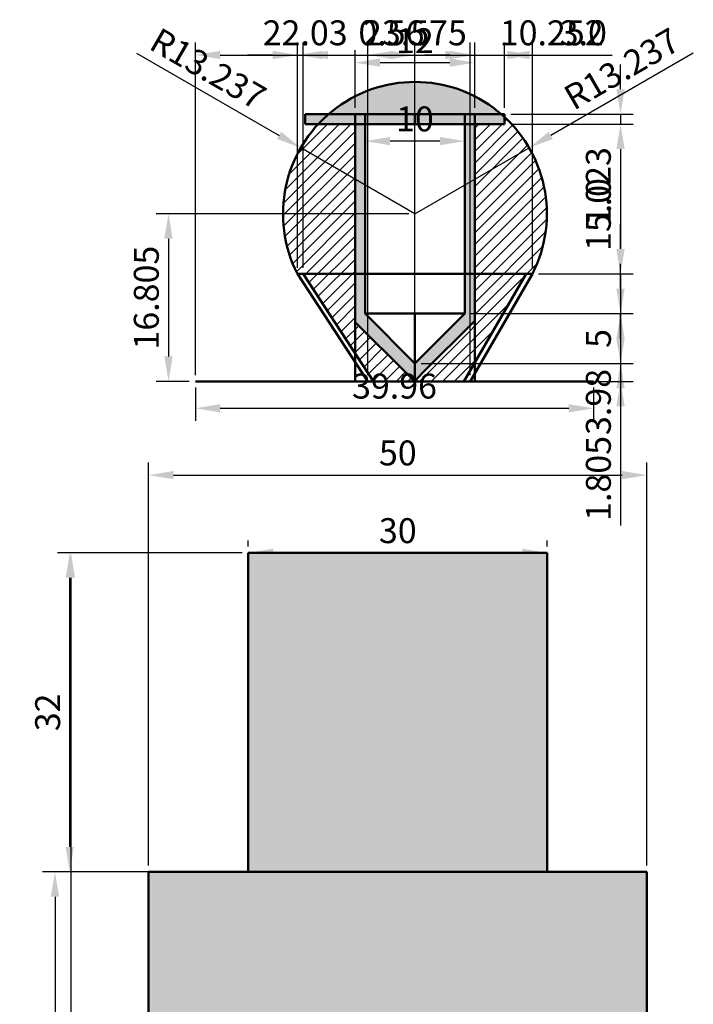
# Model space of a CAD drawing. Units: millimetres. Extents: x 1159 to 1466, y 1237 to 1440.
# Tile 2 of 6: x 1163 to 1230, y 1341 to 1440. Entities that reach past the tile are written whole.
import ezdxf

# ---------------------------------------------------------------- set-up
doc = ezdxf.new("R2010")
doc.units = ezdxf.units.MM
for name, color, linetype, lineweight in [('M-DIMS', 2, 'Continuous', 25), ('M-HATC', 8, 'Continuous', 18), ('M-OUTL', 7, 'Continuous', 50)]:
    doc.layers.add(name, color=color, linetype=linetype, lineweight=lineweight)
doc.styles.get("Standard").update_dxf_attribs({"font": 'arial.ttf'})
doc.dimstyles.new('ISO-25', dxfattribs={"dimtxt": 2.5, "dimasz": 2.5, "dimexe": 1.25, "dimexo": 0.625, "dimtad": 1, "dimtxsty": 'Standard', "dimcen": 2.5, "dimadec": 0, "dimazin": 0, "dimtfac": 1, "dimtmove": 0, "dimatfit": 3, "dimfxl": 1, "dimarcsym": 0})

# ---------------------------------------------------------------- blocks, each defined once
blk = doc.blocks.new('*D2')
at = {"layer": 'Defpoints', "color": 0, "transparency": 16777216}
for p in [(1208.23, 1435.45), (1196.23, 1430.28), (1208.23, 1430.28)]:
    blk.add_point(p, dxfattribs=at)
at = {"layer": 'M-DIMS', "color": 0, "lineweight": -2, "transparency": 16777216}
for p, q in [((1196.23, 1430.905), (1196.23, 1436.7)), ((1208.23, 1430.905), (1208.23, 1436.7)), ((1198.73, 1435.45), (1205.73, 1435.45))]:
    blk.add_line(p, q, dxfattribs=at)
at = {"layer": 'M-DIMS', "color": 0, "transparency": 16777216}
for points in [[(1198.73, 1435.867), (1198.73, 1435.034), (1196.23, 1435.45)], [(1205.73, 1435.867), (1205.73, 1435.034), (1208.23, 1435.45)]]:
    blk.add_solid(points, dxfattribs=at)
at = {"layer": 'M-DIMS', "color": 0, "transparency": 16777216, "insert": (1202.23, 1437.33), "char_height": 2.5, "attachment_point": 5}
blk.add_mtext('12', dxfattribs=at)
blk = doc.blocks.new('*D9')
at = {"layer": 'Defpoints', "color": 0, "transparency": 16777216}
for p in [(1185.51, 1386.27), (1215.51, 1386.27), (1215.51, 1386.27)]:
    blk.add_point(p, dxfattribs=at)
at = {"layer": 'M-DIMS', "color": 0, "lineweight": -2, "transparency": 16777216}
for p, q in [((1185.51, 1386.895), (1185.51, 1387.52)), ((1215.51, 1386.895), (1215.51, 1387.52)), ((1188.01, 1386.27), (1213.01, 1386.27))]:
    blk.add_line(p, q, dxfattribs=at)
at = {"layer": 'M-DIMS', "color": 0, "transparency": 16777216}
for points in [[(1188.01, 1386.687), (1188.01, 1385.854), (1185.51, 1386.27)], [(1213.01, 1386.687), (1213.01, 1385.854), (1215.51, 1386.27)]]:
    blk.add_solid(points, dxfattribs=at)
at = {"layer": 'M-DIMS', "color": 0, "transparency": 16777216, "insert": (1200.51, 1388.173), "char_height": 2.5, "attachment_point": 5}
blk.add_mtext('30', dxfattribs=at)
blk = doc.blocks.new('*D11')
at = {"layer": 'Defpoints', "color": 0, "transparency": 16777216}
for p in [(1167.601, 1386.27), (1185.51, 1386.27), (1185.51, 1354.27)]:
    blk.add_point(p, dxfattribs=at)
at = {"layer": 'M-DIMS', "color": 0, "lineweight": -2, "transparency": 16777216}
for p, q in [((1184.885, 1386.27), (1166.351, 1386.27)), ((1167.601, 1356.77), (1167.601, 1383.77)), ((1184.885, 1354.27), (1166.351, 1354.27))]:
    blk.add_line(p, q, dxfattribs=at)
at = {"layer": 'M-DIMS', "color": 0, "transparency": 16777216}
for points in [[(1167.185, 1383.77), (1168.018, 1383.77), (1167.601, 1386.27)], [(1167.185, 1356.77), (1168.018, 1356.77), (1167.601, 1354.27)]]:
    blk.add_solid(points, dxfattribs=at)
at = {"layer": 'M-DIMS', "color": 0, "transparency": 16777216, "insert": (1165.699, 1370.27), "char_height": 2.5, "attachment_point": 5, "rotation": 90}
blk.add_mtext('32', dxfattribs=at)
blk = doc.blocks.new('*D12')
at = {"layer": 'Defpoints', "color": 0, "transparency": 16777216}
for p in [(1175.51, 1354.27), (1166.114, 1320.27), (1175.51, 1320.27)]:
    blk.add_point(p, dxfattribs=at)
at = {"layer": 'M-DIMS', "color": 0, "lineweight": -2, "transparency": 16777216}
for p, q in [((1174.885, 1354.27), (1164.864, 1354.27)), ((1166.114, 1351.77), (1166.114, 1322.77)), ((1174.885, 1320.27), (1164.864, 1320.27))]:
    blk.add_line(p, q, dxfattribs=at)
at = {"layer": 'M-DIMS', "color": 0, "transparency": 16777216}
for points in [[(1165.697, 1351.77), (1166.53, 1351.77), (1166.114, 1354.27)], [(1165.697, 1322.77), (1166.53, 1322.77), (1166.114, 1320.27)]]:
    blk.add_solid(points, dxfattribs=at)
at = {"layer": 'M-DIMS', "color": 0, "transparency": 16777216, "insert": (1164.211, 1337.27), "char_height": 2.5, "attachment_point": 5, "rotation": 90}
blk.add_mtext('34', dxfattribs=at)
blk = doc.blocks.new('*D23')
at = {"layer": 'Defpoints', "color": 0, "transparency": 16777216}
for p in [(1185.51, 1386.27), (1167.71, 1260.27), (1190.51, 1260.27)]:
    blk.add_point(p, dxfattribs=at)
at = {"layer": 'M-DIMS', "color": 0, "lineweight": -2, "transparency": 16777216}
for p, q in [((1184.885, 1386.27), (1166.46, 1386.27)), ((1167.71, 1383.77), (1167.71, 1262.77)), ((1189.885, 1260.27), (1166.46, 1260.27))]:
    blk.add_line(p, q, dxfattribs=at)
at = {"layer": 'M-DIMS', "color": 0, "transparency": 16777216}
for points in [[(1167.293, 1383.77), (1168.127, 1383.77), (1167.71, 1386.27)], [(1167.293, 1262.77), (1168.127, 1262.77), (1167.71, 1260.27)]]:
    blk.add_solid(points, dxfattribs=at)
at = {"layer": 'M-DIMS', "color": 0, "transparency": 16777216, "insert": (1165.809, 1323.27), "char_height": 2.5, "attachment_point": 5, "rotation": 90}
blk.add_mtext('126', dxfattribs=at)
blk = doc.blocks.new('*D24')
at = {"layer": 'Defpoints', "color": 0, "transparency": 16777216}
for p in [(1225.51, 1394.07), (1175.51, 1354.27), (1225.51, 1354.27)]:
    blk.add_point(p, dxfattribs=at)
at = {"layer": 'M-DIMS', "color": 0, "lineweight": -2, "transparency": 16777216}
for p, q in [((1175.51, 1354.895), (1175.51, 1395.32)), ((1225.51, 1354.895), (1225.51, 1395.32)), ((1178.01, 1394.07), (1223.01, 1394.07))]:
    blk.add_line(p, q, dxfattribs=at)
at = {"layer": 'M-DIMS', "color": 0, "transparency": 16777216}
for points in [[(1178.01, 1394.487), (1178.01, 1393.654), (1175.51, 1394.07)], [(1223.01, 1394.487), (1223.01, 1393.654), (1225.51, 1394.07)]]:
    blk.add_solid(points, dxfattribs=at)
at = {"layer": 'M-DIMS', "color": 0, "transparency": 16777216, "insert": (1200.51, 1395.972), "char_height": 2.5, "attachment_point": 5}
blk.add_mtext('50', dxfattribs=at)
blk = doc.blocks.new('*D37')
at = {"layer": 'Defpoints', "color": 0, "transparency": 16777216}
for p in [(1202.23, 1420.28), (1177.501, 1403.475), (1180.201, 1403.475)]:
    blk.add_point(p, dxfattribs=at)
at = {"layer": 'M-DIMS', "color": 0, "lineweight": -2, "transparency": 16777216}
for p, q in [((1201.605, 1420.28), (1176.251, 1420.28)), ((1177.501, 1417.78), (1177.501, 1405.975)), ((1179.576, 1403.475), (1176.251, 1403.475))]:
    blk.add_line(p, q, dxfattribs=at)
at = {"layer": 'M-DIMS', "color": 0, "transparency": 16777216}
for points in [[(1177.085, 1417.78), (1177.918, 1417.78), (1177.501, 1420.28)], [(1177.085, 1405.975), (1177.918, 1405.975), (1177.501, 1403.475)]]:
    blk.add_solid(points, dxfattribs=at)
at = {"layer": 'M-DIMS', "color": 0, "transparency": 16777216, "insert": (1175.6, 1411.877), "char_height": 2.5, "attachment_point": 5, "rotation": 90}
blk.add_mtext('16.805', dxfattribs=at)
blk = doc.blocks.new('*D38')
at = {"layer": 'Defpoints', "color": 0, "transparency": 16777216}
for p in [(1180.201, 1403.475), (1220.161, 1403.475), (1220.161, 1400.775)]:
    blk.add_point(p, dxfattribs=at)
at = {"layer": 'M-DIMS', "color": 0, "lineweight": -2, "transparency": 16777216}
for p, q in [((1180.201, 1402.85), (1180.201, 1399.525)), ((1220.161, 1402.85), (1220.161, 1399.525)), ((1182.701, 1400.775), (1217.661, 1400.775))]:
    blk.add_line(p, q, dxfattribs=at)
at = {"layer": 'M-DIMS', "color": 0, "transparency": 16777216}
for points in [[(1182.701, 1401.192), (1182.701, 1400.358), (1180.201, 1400.775)], [(1217.661, 1401.192), (1217.661, 1400.358), (1220.161, 1400.775)]]:
    blk.add_solid(points, dxfattribs=at)
at = {"layer": 'M-DIMS', "color": 0, "transparency": 16777216, "insert": (1200.181, 1402.677), "char_height": 2.5, "attachment_point": 5}
blk.add_mtext('39.96', dxfattribs=at)
blk = doc.blocks.new('*D39')
at = {"layer": 'Defpoints', "color": 0, "transparency": 16777216}
for p in [(1197.23, 1430.28), (1207.23, 1430.28), (1197.23, 1427.58)]:
    blk.add_point(p, dxfattribs=at)
at = {"layer": 'M-DIMS', "color": 0, "lineweight": -2, "transparency": 16777216}
for p, q in [((1197.23, 1429.655), (1197.23, 1426.33)), ((1207.23, 1429.655), (1207.23, 1426.33)), ((1204.73, 1427.58), (1199.73, 1427.58))]:
    blk.add_line(p, q, dxfattribs=at)
at = {"layer": 'M-DIMS', "color": 0, "transparency": 16777216}
for points in [[(1199.73, 1427.997), (1199.73, 1427.163), (1197.23, 1427.58)], [(1204.73, 1427.997), (1204.73, 1427.163), (1207.23, 1427.58)]]:
    blk.add_solid(points, dxfattribs=at)
at = {"layer": 'M-DIMS', "color": 0, "transparency": 16777216, "insert": (1202.23, 1429.481), "char_height": 2.5, "attachment_point": 5}
blk.add_mtext('10', dxfattribs=at)
blk = doc.blocks.new('*D40')
at = {"layer": 'Defpoints', "color": 0, "transparency": 16777216}
for p in [(1207.23, 1410.28), (1202.23, 1405.28), (1222.861, 1405.28)]:
    blk.add_point(p, dxfattribs=at)
at = {"layer": 'M-DIMS', "color": 0, "lineweight": -2, "transparency": 16777216}
for p, q in [((1222.861, 1412.78), (1222.861, 1415.28)), ((1207.855, 1410.28), (1224.111, 1410.28)), ((1222.861, 1410.28), (1222.861, 1405.28)), ((1202.855, 1405.28), (1224.111, 1405.28)), ((1222.861, 1402.78), (1222.861, 1400.28))]:
    blk.add_line(p, q, dxfattribs=at)
at = {"layer": 'M-DIMS', "color": 0, "transparency": 16777216}
for points in [[(1222.444, 1412.78), (1223.277, 1412.78), (1222.861, 1410.28)], [(1222.444, 1402.78), (1223.277, 1402.78), (1222.861, 1405.28)]]:
    blk.add_solid(points, dxfattribs=at)
at = {"layer": 'M-DIMS', "color": 0, "transparency": 16777216, "insert": (1220.964, 1407.78), "char_height": 2.5, "attachment_point": 5, "rotation": 90}
blk.add_mtext('5', dxfattribs=at)
blk = doc.blocks.new('*D52')
at = {"layer": 'Defpoints', "color": 0, "transparency": 16777216}
for p in [(1190.768, 1426.901), (1202.23, 1420.28)]:
    blk.add_point(p, dxfattribs=at)
at = {"layer": 'M-DIMS', "color": 0, "lineweight": -2, "transparency": 16777216}
for p, q in [((1174.297, 1436.416), (1188.603, 1428.152)), ((1202.23, 1420.28), (1190.768, 1426.901))]:
    blk.add_line(p, q, dxfattribs=at)
at = {"layer": 'M-DIMS', "color": 0, "transparency": 16777216}
blk.add_solid([(1188.811, 1428.513), (1188.394, 1427.791), (1190.768, 1426.901)], dxfattribs=at)
at = {"layer": 'M-DIMS', "color": 0, "transparency": 16777216, "insert": (1181.319, 1434.556), "char_height": 2.5, "attachment_point": 5, "rotation": 329.98548}
blk.add_mtext('R13.237', dxfattribs=at)
blk = doc.blocks.new('*D79')
at = {"layer": 'Defpoints', "color": 0, "transparency": 16777216}
for p in [(1211.23, 1436.217), (1208.23, 1430.28), (1211.23, 1430.28)]:
    blk.add_point(p, dxfattribs=at)
at = {"layer": 'M-DIMS', "color": 0, "lineweight": -2, "transparency": 16777216}
for p, q in [((1208.23, 1430.905), (1208.23, 1437.467)), ((1211.23, 1430.905), (1211.23, 1437.467)), ((1205.73, 1436.217), (1203.23, 1436.217)), ((1208.23, 1436.217), (1211.23, 1436.217)), ((1213.73, 1436.217), (1222.021, 1436.217))]:
    blk.add_line(p, q, dxfattribs=at)
at = {"layer": 'M-DIMS', "color": 0, "transparency": 16777216}
for points in [[(1205.73, 1436.634), (1205.73, 1435.8), (1208.23, 1436.217)], [(1213.73, 1436.634), (1213.73, 1435.8), (1211.23, 1436.217)]]:
    blk.add_solid(points, dxfattribs=at)
at = {"layer": 'M-DIMS', "color": 0, "transparency": 16777216, "insert": (1219.125, 1438.119), "char_height": 2.5, "attachment_point": 5}
blk.add_mtext('3.0', dxfattribs=at)
blk = doc.blocks.new('*D80')
at = {"layer": 'Defpoints', "color": 0, "transparency": 16777216}
for p in [(1211.23, 1430.28), (1211.23, 1429.28), (1222.861, 1429.28)]:
    blk.add_point(p, dxfattribs=at)
at = {"layer": 'M-DIMS', "color": 0, "lineweight": -2, "transparency": 16777216}
for p, q in [((1222.861, 1432.78), (1222.861, 1435.28)), ((1211.855, 1430.28), (1224.111, 1430.28)), ((1222.861, 1430.28), (1222.861, 1429.28)), ((1211.855, 1429.28), (1224.111, 1429.28)), ((1222.861, 1426.78), (1222.861, 1418.722))]:
    blk.add_line(p, q, dxfattribs=at)
at = {"layer": 'M-DIMS', "color": 0, "transparency": 16777216}
for points in [[(1222.444, 1432.78), (1223.277, 1432.78), (1222.861, 1430.28)], [(1222.444, 1426.78), (1223.277, 1426.78), (1222.861, 1429.28)]]:
    blk.add_solid(points, dxfattribs=at)
at = {"layer": 'M-DIMS', "color": 0, "transparency": 16777216, "insert": (1220.959, 1421.501), "char_height": 2.5, "attachment_point": 5, "rotation": 90}
blk.add_mtext('1.0', dxfattribs=at)
blk = doc.blocks.new('*D81')
at = {"layer": 'Defpoints', "color": 0, "transparency": 16777216}
for p in [(1211.23, 1429.28), (1214.017, 1414.256), (1222.861, 1414.256)]:
    blk.add_point(p, dxfattribs=at)
at = {"layer": 'M-DIMS', "color": 0, "lineweight": -2, "transparency": 16777216}
for p, q in [((1211.855, 1429.28), (1224.111, 1429.28)), ((1222.861, 1426.78), (1222.861, 1416.756)), ((1214.642, 1414.256), (1224.111, 1414.256))]:
    blk.add_line(p, q, dxfattribs=at)
at = {"layer": 'M-DIMS', "color": 0, "transparency": 16777216}
for points in [[(1222.444, 1426.78), (1223.277, 1426.78), (1222.861, 1429.28)], [(1222.444, 1416.756), (1223.277, 1416.756), (1222.861, 1414.256)]]:
    blk.add_solid(points, dxfattribs=at)
at = {"layer": 'M-DIMS', "color": 0, "transparency": 16777216, "insert": (1220.958, 1421.768), "char_height": 2.5, "attachment_point": 5, "rotation": 90}
blk.add_mtext('15.023', dxfattribs=at)
blk = doc.blocks.new('*D82')
at = {"layer": 'Defpoints', "color": 0, "transparency": 16777216}
for p in [(1214.017, 1414.256), (1207.23, 1410.28), (1222.861, 1410.28)]:
    blk.add_point(p, dxfattribs=at)
at = {"layer": 'M-DIMS', "color": 0, "lineweight": -2, "transparency": 16777216}
for p, q in [((1222.861, 1416.756), (1222.861, 1419.256)), ((1214.642, 1414.256), (1224.111, 1414.256)), ((1222.861, 1414.256), (1222.861, 1410.28)), ((1207.855, 1410.28), (1224.111, 1410.28)), ((1222.861, 1407.78), (1222.861, 1397.533))]:
    blk.add_line(p, q, dxfattribs=at)
at = {"layer": 'M-DIMS', "color": 0, "transparency": 16777216}
for points in [[(1222.444, 1416.756), (1223.277, 1416.756), (1222.861, 1414.256)], [(1222.444, 1407.78), (1223.277, 1407.78), (1222.861, 1410.28)]]:
    blk.add_solid(points, dxfattribs=at)
at = {"layer": 'M-DIMS', "color": 0, "transparency": 16777216, "insert": (1220.958, 1401.406), "char_height": 2.5, "attachment_point": 5, "rotation": 90}
blk.add_mtext('3.98', dxfattribs=at)
blk = doc.blocks.new('*D83')
at = {"layer": 'Defpoints', "color": 0, "transparency": 16777216}
for p in [(1202.23, 1405.28), (1220.161, 1403.475), (1222.861, 1403.475)]:
    blk.add_point(p, dxfattribs=at)
at = {"layer": 'M-DIMS', "color": 0, "lineweight": -2, "transparency": 16777216}
for p, q in [((1222.861, 1407.78), (1222.861, 1410.28)), ((1202.855, 1405.28), (1224.111, 1405.28)), ((1222.861, 1405.28), (1222.861, 1403.475)), ((1220.786, 1403.475), (1224.111, 1403.475)), ((1222.861, 1400.975), (1222.861, 1389.005))]:
    blk.add_line(p, q, dxfattribs=at)
at = {"layer": 'M-DIMS', "color": 0, "transparency": 16777216}
for points in [[(1222.444, 1407.78), (1223.277, 1407.78), (1222.861, 1405.28)], [(1222.444, 1400.975), (1223.277, 1400.975), (1222.861, 1403.475)]]:
    blk.add_solid(points, dxfattribs=at)
at = {"layer": 'M-DIMS', "color": 0, "transparency": 16777216, "insert": (1220.959, 1393.74), "char_height": 2.5, "attachment_point": 5, "rotation": 90}
blk.add_mtext('1.805', dxfattribs=at)
blk = doc.blocks.new('*D84')
at = {"layer": 'Defpoints', "color": 0, "transparency": 16777216}
for p in [(1202.23, 1436.217), (1202.23, 1405.28), (1180.201, 1403.475)]:
    blk.add_point(p, dxfattribs=at)
at = {"layer": 'M-DIMS', "color": 0, "lineweight": -2, "transparency": 16777216}
for p, q in [((1180.201, 1404.1), (1180.201, 1437.467)), ((1202.23, 1405.905), (1202.23, 1437.467)), ((1182.701, 1436.217), (1199.73, 1436.217))]:
    blk.add_line(p, q, dxfattribs=at)
at = {"layer": 'M-DIMS', "color": 0, "transparency": 16777216}
for points in [[(1182.701, 1436.634), (1182.701, 1435.8), (1180.201, 1436.217)], [(1199.73, 1436.634), (1199.73, 1435.8), (1202.23, 1436.217)]]:
    blk.add_solid(points, dxfattribs=at)
at = {"layer": 'M-DIMS', "color": 0, "transparency": 16777216, "insert": (1191.216, 1438.119), "char_height": 2.5, "attachment_point": 5}
blk.add_mtext('22.03', dxfattribs=at)
blk = doc.blocks.new('*D85')
at = {"layer": 'Defpoints', "color": 0, "transparency": 16777216}
for p in [(1214.017, 1436.217), (1190.442, 1414.256), (1214.017, 1414.256)]:
    blk.add_point(p, dxfattribs=at)
at = {"layer": 'M-DIMS', "color": 0, "lineweight": -2, "transparency": 16777216}
for p, q in [((1190.442, 1414.881), (1190.442, 1437.467)), ((1214.017, 1414.881), (1214.017, 1437.467)), ((1192.942, 1436.217), (1211.517, 1436.217))]:
    blk.add_line(p, q, dxfattribs=at)
at = {"layer": 'M-DIMS', "color": 0, "transparency": 16777216}
for points in [[(1192.942, 1436.634), (1192.942, 1435.8), (1190.442, 1436.217)], [(1211.517, 1436.634), (1211.517, 1435.8), (1214.017, 1436.217)]]:
    blk.add_solid(points, dxfattribs=at)
at = {"layer": 'M-DIMS', "color": 0, "transparency": 16777216, "insert": (1202.23, 1438.119), "char_height": 2.5, "attachment_point": 5}
blk.add_mtext('23.575', dxfattribs=at)
blk = doc.blocks.new('*D86')
at = {"layer": 'Defpoints', "color": 0, "transparency": 16777216}
for p in [(1207.768, 1436.217), (1197.516, 1403.475), (1207.768, 1403.475)]:
    blk.add_point(p, dxfattribs=at)
at = {"layer": 'M-DIMS', "color": 0, "lineweight": -2, "transparency": 16777216}
for p, q in [((1197.516, 1404.1), (1197.516, 1437.467)), ((1207.768, 1404.1), (1207.768, 1437.467)), ((1200.016, 1436.217), (1205.268, 1436.217)), ((1207.768, 1436.217), (1221.636, 1436.217))]:
    blk.add_line(p, q, dxfattribs=at)
at = {"layer": 'M-DIMS', "color": 0, "transparency": 16777216}
for points in [[(1200.016, 1436.634), (1200.016, 1435.8), (1197.516, 1436.217)], [(1205.268, 1436.634), (1205.268, 1435.8), (1207.768, 1436.217)]]:
    blk.add_solid(points, dxfattribs=at)
at = {"layer": 'M-DIMS', "color": 0, "transparency": 16777216, "insert": (1215.952, 1438.119), "char_height": 2.5, "attachment_point": 5}
blk.add_mtext('10.252', dxfattribs=at)
blk = doc.blocks.new('*D87')
at = {"layer": 'Defpoints', "color": 0, "transparency": 16777216}
for p in [(1191.001, 1436.217), (1190.442, 1414.256), (1191.001, 1414.256)]:
    blk.add_point(p, dxfattribs=at)
at = {"layer": 'M-DIMS', "color": 0, "lineweight": -2, "transparency": 16777216}
for p, q in [((1190.442, 1414.881), (1190.442, 1437.467)), ((1191.001, 1414.881), (1191.001, 1437.467)), ((1187.942, 1436.217), (1185.442, 1436.217)), ((1190.442, 1436.217), (1191.001, 1436.217)), ((1193.501, 1436.217), (1203.743, 1436.217))]:
    blk.add_line(p, q, dxfattribs=at)
at = {"layer": 'M-DIMS', "color": 0, "transparency": 16777216}
for points in [[(1187.942, 1436.634), (1187.942, 1435.8), (1190.442, 1436.217)], [(1193.501, 1436.634), (1193.501, 1435.8), (1191.001, 1436.217)]]:
    blk.add_solid(points, dxfattribs=at)
at = {"layer": 'M-DIMS', "color": 0, "transparency": 16777216, "insert": (1199.872, 1438.119), "char_height": 2.5, "attachment_point": 5}
blk.add_mtext('0.56', dxfattribs=at)
blk = doc.blocks.new('*D91')
at = {"layer": 'Defpoints', "color": 0, "transparency": 16777216}
for p in [(1213.692, 1426.901), (1202.23, 1420.28)]:
    blk.add_point(p, dxfattribs=at)
at = {"layer": 'M-DIMS', "color": 0, "lineweight": -2, "transparency": 16777216}
for p, q in [((1230.163, 1436.415), (1215.857, 1428.152)), ((1202.23, 1420.28), (1213.692, 1426.901))]:
    blk.add_line(p, q, dxfattribs=at)
at = {"layer": 'M-DIMS', "color": 0, "transparency": 16777216}
blk.add_solid([(1215.648, 1428.512), (1216.065, 1427.791), (1213.692, 1426.901)], dxfattribs=at)
at = {"layer": 'M-DIMS', "color": 0, "transparency": 16777216, "insert": (1223.14, 1434.556), "char_height": 2.5, "attachment_point": 5, "rotation": 30.0131}
blk.add_mtext('R13.237', dxfattribs=at)

msp = doc.modelspace()

# ---------------------------------------------------------------- hatches: boundary and pattern name
at = {"layer": 'M-HATC'}
h = msp.add_hatch(color=256, dxfattribs=at)
h.set_gradient(color1=(99, 100, 102))
h.paths.add_polyline_path([(1207.2297, 1430.2799), (1208.2297, 1430.2799), (1210.9028, 1430.2799, 0.3732444), (1193.5565, 1430.2799), (1196.2297, 1430.2799), (1197.2297, 1430.2799)])
h = msp.add_hatch(dxfattribs=at)
h.set_pattern_fill('ANSI31', color=256, scale=0.26)
h.paths.add_polyline_path([(1196.2297, 1429.2799), (1192.5228, 1429.2799, 0.3148356), (1190.4423, 1414.2564), (1196.2297, 1414.2564)])
h.paths.add_polyline_path([(1211.2297, 1429.9868), (1211.2297, 1429.2799), (1208.2297, 1429.2799), (1208.2297, 1414.2564), (1214.017, 1414.2564, 0.3357189)])
h.paths.add_polyline_path([(1213.3979, 1414.2564), (1208.2297, 1414.2564), (1208.2297, 1410.2799), (1208.2297, 1409.5577), (1208.2297, 1405.3395)])
h.paths.add_polyline_path([(1208.2297, 1405.3395), (1208.2297, 1409.5577), (1208.0936, 1409.4159), (1203.0936, 1404.4159), (1202.1793, 1403.4749), (1207.149, 1403.4749)])
h.paths.add_polyline_path([(1196.3014, 1409.3516), (1196.2297, 1409.4295), (1196.2297, 1406.2872), (1198.0747, 1403.4749), (1202.1793, 1403.4749), (1201.3014, 1404.3516)])
h.paths.add_polyline_path([(1196.2297, 1414.2564), (1191.0011, 1414.2564), (1196.2297, 1406.2872), (1196.2297, 1409.4295), (1196.2297, 1410.2799)])
h = msp.add_hatch(color=256, dxfattribs=at)
h.set_gradient(color1=(244, 238, 81))
h.paths.add_polyline_path([(1202.2297, 1430.2799), (1197.2297, 1430.2799), (1197.2297, 1429.2799), (1202.2297, 1429.2799)])
h.paths.add_polyline_path([(1207.2297, 1430.2799), (1202.2297, 1430.2799), (1202.2297, 1429.2799), (1207.2297, 1429.2799)])
h.paths.add_polyline_path([(1208.2297, 1430.2799), (1207.2297, 1430.2799), (1207.2297, 1429.2799), (1208.2297, 1429.2799)])
h.paths.add_polyline_path([(1211.2297, 1429.9868, 0.0082921), (1210.9028, 1430.2799), (1208.2297, 1430.2799), (1208.2297, 1429.2799), (1211.2297, 1429.2799)])
h.paths.add_polyline_path([(1193.5565, 1430.2799), (1191.2297, 1430.2799), (1191.2297, 1429.2799), (1192.5228, 1429.2799, -0.0271833)])
h.paths.add_polyline_path([(1196.2297, 1430.2799), (1193.5565, 1430.2799, 0.0271833), (1192.5228, 1429.2799), (1196.2297, 1429.2799)])
h.paths.add_polyline_path([(1197.2297, 1430.2799), (1196.2297, 1430.2799), (1196.2297, 1429.2799), (1197.2297, 1429.2799)])
h = msp.add_hatch(color=256, dxfattribs=at)
h.set_gradient(color1=(205, 32, 39))
h.paths.add_polyline_path([(1197.2297, 1429.2799), (1196.2297, 1429.2799), (1196.2297, 1414.2564), (1197.2297, 1414.2564)])
h.paths.add_polyline_path([(1208.2297, 1429.2799), (1207.2297, 1429.2799), (1207.2297, 1414.2564), (1208.2297, 1414.2564)])
h.paths.add_polyline_path([(1197.2297, 1414.2564), (1196.2297, 1414.2564), (1196.2297, 1410.2799), (1196.2297, 1409.4295), (1196.3014, 1409.3516), (1201.3014, 1404.3516), (1202.1793, 1403.4749), (1202.2297, 1403.5268), (1202.2297, 1405.2799), (1197.2297, 1410.2799)])
h.paths.add_polyline_path([(1208.0936, 1409.4159), (1208.2297, 1409.5577), (1208.2297, 1410.2799), (1208.2297, 1414.2564), (1207.2297, 1414.2564), (1207.2297, 1410.2799), (1202.2297, 1405.2799), (1202.2297, 1403.5268), (1203.0936, 1404.4159)])
h = msp.add_hatch(color=256, dxfattribs=at)
h.set_gradient(color1=(254, 204, 102), color2=(254, 204, 102))
h.paths.add_polyline_path([(1215.5099, 1386.2704), (1185.5099, 1386.2704), (1185.5099, 1354.2704), (1215.5099, 1354.2704)])
h.paths.add_polyline_path([(1225.5099, 1354.2704), (1215.5099, 1354.2704), (1185.5099, 1354.2704), (1175.5099, 1354.2704), (1175.5099, 1320.2704), (1178.0099, 1320.2704), (1223.0099, 1320.2704), (1225.5099, 1320.2704)])
h.paths.add_polyline_path([(1200.5099, 1270.2704), (1180.5099, 1270.2704), (1190.5099, 1260.2704), (1200.5099, 1260.2704)])
h.paths.add_polyline_path([(1220.5099, 1270.2704), (1200.5099, 1270.2704), (1200.5099, 1260.2704), (1210.5099, 1260.2704)])

# ---------------------------------------------------------------- linework, layer by layer
at = {"layer": 'M-OUTL'}
for p, q in [((1196.2297, 1430.2799), (1191.2297, 1430.2799)), ((1191.2297, 1430.2799), (1191.2297, 1429.2799)), ((1197.2297, 1430.2799), (1196.2297, 1430.2799)), ((1196.2297, 1430.2799), (1196.2297, 1410.2799)), ((1197.2297, 1430.2799), (1207.2297, 1430.2799)), ((1197.2297, 1410.2799), (1197.2297, 1430.2799)), ((1202.2297, 1430.2799), (1202.2297, 1429.2799)), ((1207.2297, 1430.2799), (1207.2297, 1410.2799)), ((1207.2297, 1430.2799), (1208.2297, 1430.2799)), ((1208.2297, 1430.2799), (1208.2297, 1410.2799)), ((1211.2297, 1430.2799), (1208.2297, 1430.2799)), ((1211.2297, 1429.2799), (1211.2297, 1430.2799)), ((1191.2297, 1429.2799), (1211.2297, 1429.2799)), ((1190.4423, 1414.2564), (1214.017, 1414.2564)), ((1190.4423, 1414.2564), (1197.5159, 1403.4749)), ((1191.0011, 1414.2564), (1198.0747, 1403.4749)), ((1213.3979, 1414.2564), (1207.149, 1403.4749)), ((1214.017, 1414.2564), (1207.7681, 1403.4749)), ((1196.2297, 1410.2799), (1196.2297, 1409.4295)), ((1207.2297, 1410.2799), (1197.2297, 1410.2799)), ((1197.2297, 1410.2799), (1202.2297, 1405.2799)), ((1202.2297, 1410.2799), (1202.2297, 1405.2799)), ((1202.2297, 1405.2799), (1207.2297, 1410.2799)), ((1208.2297, 1410.2799), (1208.2297, 1409.5577)), ((1196.3014, 1409.3516), (1196.2297, 1409.4295)), ((1196.2297, 1409.4295), (1196.2297, 1403.4749)), ((1196.3014, 1409.3516), (1201.3014, 1404.3516)), ((1203.0936, 1404.4159), (1208.0936, 1409.4159)), ((1208.0936, 1409.4159), (1208.2297, 1409.5577)), ((1208.2297, 1409.5577), (1208.2297, 1403.4749)), ((1202.2297, 1405.2799), (1202.2297, 1403.5268)), ((1201.3014, 1404.3516), (1202.1793, 1403.4749)), ((1203.0936, 1404.4159), (1202.1793, 1403.4749)), ((1202.1793, 1403.4749), (1180.2014, 1403.4749)), ((1202.1793, 1403.4749), (1220.1607, 1403.4749)), ((1185.5099, 1386.2704), (1215.5099, 1386.2704)), ((1185.5099, 1354.2704), (1185.5099, 1386.2704)), ((1215.5099, 1386.2704), (1215.5099, 1354.2704)), ((1185.5099, 1354.2704), (1175.5099, 1354.2704)), ((1175.5099, 1354.2704), (1175.5099, 1320.2704)), ((1215.5099, 1354.2704), (1185.5099, 1354.2704)), ((1225.5099, 1354.2704), (1215.5099, 1354.2704)), ((1225.5099, 1320.2704), (1225.5099, 1354.2704))]:
    msp.add_line(p, q, dxfattribs=at)
msp.add_arc((1202.2297, 1420.2799), 13.2372, 332.932536, 207.067464, dxfattribs=at)

# ---------------------------------------------------------------- dimensions: what is measured, and where the dimension line sits
at = {"layer": 'M-DIMS'}
for base, p1, p2, override, picture, middle in [((1202.2297, 1436.2171), (1180.2014, 1403.4749), (1202.2297, 1405.2799), {"dimdec": 2, "dimlfac": 1, "dimrnd": 0, "dimzin": 0, "dimdsep": 46, "dimlunit": 2}, '*D84', (1191.2155, 1438.1194)), ((1191.0011, 1436.2171), (1190.4423, 1414.2564), (1191.0011, 1414.2564), {"dimdec": 2, "dimlfac": 1, "dimrnd": 0, "dimzin": 0, "dimdsep": 46, "dimlunit": 2}, '*D87', (1199.8722, 1438.1185)), ((1214.017, 1436.2171), (1190.4423, 1414.2564), (1214.017, 1414.2564), {"dimdec": 3, "dimlfac": 1, "dimrnd": 0, "dimzin": 0, "dimdsep": 46, "dimlunit": 2}, '*D85', (1202.2297, 1438.1194)), ((1207.7681, 1436.2171), (1197.5159, 1403.4749), (1207.7681, 1403.4749), {"dimdec": 3, "dimlfac": 1, "dimrnd": 0, "dimzin": 0, "dimdsep": 46, "dimlunit": 2}, '*D86', (1215.9519, 1438.1185)), ((1211.2297, 1436.2171), (1208.2297, 1430.2799), (1211.2297, 1430.2799), {"dimdec": 1, "dimlfac": 1, "dimrnd": 0, "dimzin": 0, "dimdsep": 46, "dimlunit": 2}, '*D79', (1219.1253, 1438.1194)), ((1208.2297, 1435.4503), (1196.2297, 1430.2799), (1208.2297, 1430.2799), {"dimclrd": 0, "dimclre": 0, "dimclrt": 0}, '*D2', (1202.2297, 1437.3304)), ((1220.1607, 1400.7749), (1180.2014, 1403.4749), (1220.1607, 1403.4749), {"dimdec": 2, "dimlfac": 1, "dimrnd": 0, "dimzin": 0, "dimdsep": 46, "dimlunit": 2}, '*D38', (1200.181, 1402.6772)), ((1225.5099, 1394.0704), (1175.5099, 1354.2704), (1225.5099, 1354.2704), {"dimdec": 0, "dimlfac": 1, "dimrnd": 0, "dimzin": 0, "dimdsep": 46, "dimlunit": 2}, '*D24', (1200.5099, 1395.9718)), ((1215.5099, 1386.2704), (1185.5099, 1386.2704), (1215.5099, 1386.2704), {"dimclrd": 0, "dimclre": 0, "dimclrt": 0}, '*D9', (1200.5099, 1388.1727))]:
    dim = msp.add_linear_dim(base=base, p1=p1, p2=p2, dimstyle='ISO-25', override=override, dxfattribs=at)
    dim.commit()
    dim.dimension.update_dxf_attribs({"geometry": picture, "text_midpoint": middle})
for mpoint, picture, middle in [((1190.7676, 1426.9014), '*D52', (1181.3192, 1434.5565)), ((1213.6919, 1426.9011), '*D91', (1223.1405, 1434.556))]:
    dim = msp.add_radius_dim(center=(1202.2297, 1420.2799), mpoint=mpoint, dimstyle='ISO-25', override={"dimdec": 3, "dimlfac": 1, "dimrnd": 0, "dimzin": 0, "dimdsep": 46, "dimlunit": 2}, dxfattribs=at)
    dim.commit()
    dim.dimension.update_dxf_attribs({"geometry": picture, "text_midpoint": middle})
for base, p1, p2, angle, override, picture, middle in [((1222.8607, 1429.2799), (1211.2297, 1430.2799), (1211.2297, 1429.2799), 90, {"dimdec": 1, "dimlfac": 1, "dimrnd": 0, "dimzin": 0, "dimdsep": 46, "dimlunit": 2}, '*D80', (1220.9593, 1421.5011)), ((1197.2297, 1427.5799), (1207.2297, 1430.2799), (1197.2297, 1430.2799), 180, {"dimdec": 0, "dimlfac": 1, "dimrnd": 0, "dimzin": 0, "dimdsep": 46, "dimlunit": 2}, '*D39', (1202.2297, 1429.4813)), ((1222.86073, 1414.25643), (1211.22967, 1429.27988), (1214.01703, 1414.25643), 90, {"dimdec": 3, "dimlfac": 1, "dimrnd": 0, "dimzin": 0, "dimdsep": 46, "dimlunit": 2}, '*D81', (1220.95845, 1421.76816)), ((1177.5014, 1403.4749), (1202.2297, 1420.2799), (1180.2014, 1403.4749), 90, {"dimdec": 3, "dimlfac": 1, "dimrnd": 0, "dimzin": 0, "dimdsep": 46, "dimlunit": 2}, '*D37', (1175.5999, 1411.8774)), ((1222.8607, 1410.2799), (1214.017, 1414.2564), (1207.2297, 1410.2799), 90, {"dimdec": 2, "dimlfac": 1, "dimrnd": 0, "dimzin": 0, "dimdsep": 46, "dimlunit": 2}, '*D82', (1220.9584, 1401.4062)), ((1222.8607, 1405.2799), (1207.2297, 1410.2799), (1202.2297, 1405.2799), 90, {"dimdec": 0, "dimlfac": 1, "dimrnd": 0, "dimzin": 0, "dimdsep": 46, "dimlunit": 2}, '*D40', (1220.9644, 1407.7799)), ((1222.8607, 1403.4749), (1202.2297, 1405.2799), (1220.1607, 1403.4749), 90, {"dimdec": 3, "dimlfac": 1, "dimrnd": 0, "dimzin": 0, "dimdsep": 46, "dimlunit": 2}, '*D83', (1220.9593, 1393.7401)), ((1167.6015, 1386.2704), (1185.5099, 1354.2704), (1185.5099, 1386.2704), 90, {"dimclrd": 0, "dimclre": 0, "dimclrt": 0}, '*D11', (1165.6992, 1370.2704)), ((1167.7099, 1260.2704), (1185.5099, 1386.2704), (1190.5099, 1260.2704), 90, {"dimdec": 0, "dimlfac": 1, "dimrnd": 0, "dimzin": 0, "dimdsep": 46, "dimlunit": 2}, '*D23', (1165.8085, 1323.2704)), ((1166.1136, 1320.2704), (1175.5099, 1354.2704), (1175.5099, 1320.2704), 90, {"dimclrd": 0, "dimclre": 0, "dimclrt": 0}, '*D12', (1164.2113, 1337.2704))]:
    dim = msp.add_linear_dim(base=base, p1=p1, p2=p2, angle=angle, dimstyle='ISO-25', override=override, dxfattribs=at)
    dim.commit()
    dim.dimension.update_dxf_attribs({"geometry": picture, "text_midpoint": middle})

doc.saveas('drawing.dxf')
